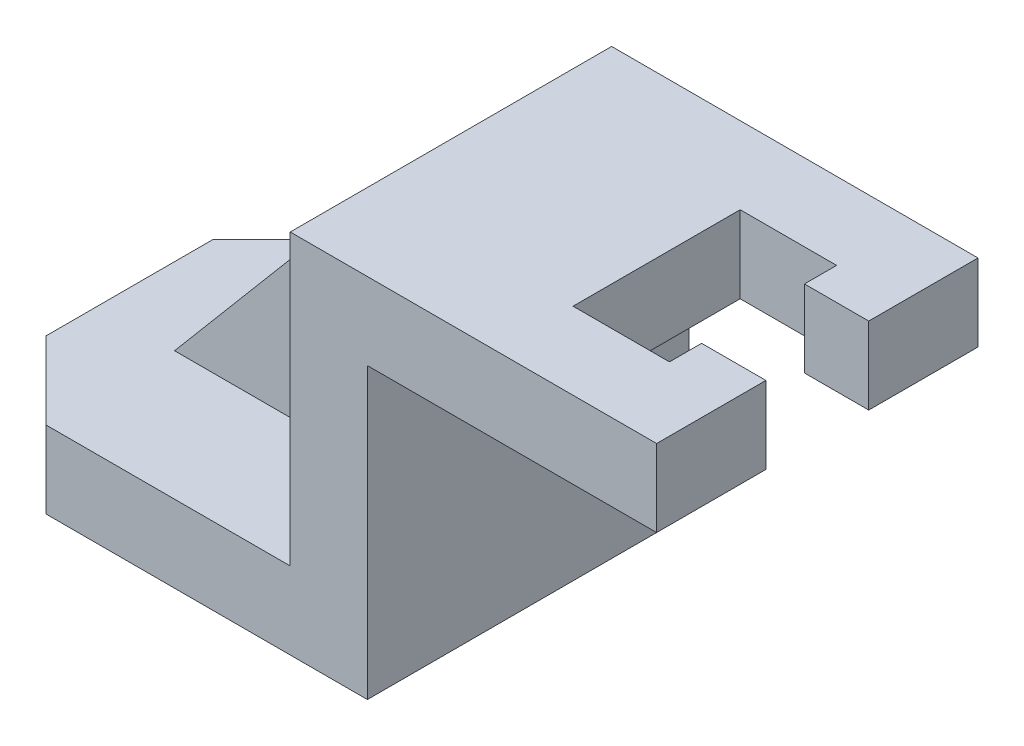
ISO-10303-21;
HEADER;
FILE_DESCRIPTION(('STEP AP214'),'2;1');
FILE_NAME('part.step','',(''),(''),'','','');
FILE_SCHEMA(('AUTOMOTIVE_DESIGN { 1 0 10303 214 1 1 1 1 }'));
ENDSEC;
DATA;
#1=APPLICATION_CONTEXT('core data for automotive mechanical design processes');
#2=APPLICATION_PROTOCOL_DEFINITION('international standard','automotive_design',2000,#1);
#3=PRODUCT_CONTEXT('',#1,'mechanical');
#4=PRODUCT('Part','Part','',(#3));
#5=PRODUCT_RELATED_PRODUCT_CATEGORY('part','',(#4));
#6=PRODUCT_DEFINITION_FORMATION('','',#4);
#7=PRODUCT_DEFINITION_CONTEXT('part definition',#1,'design');
#8=PRODUCT_DEFINITION('design','',#6,#7);
#9=PRODUCT_DEFINITION_SHAPE('','',#8);
#10=(LENGTH_UNIT() NAMED_UNIT(*) SI_UNIT(.MILLI.,.METRE.));
#11=(NAMED_UNIT(*) PLANE_ANGLE_UNIT() SI_UNIT($,.RADIAN.));
#12=(NAMED_UNIT(*) SI_UNIT($,.STERADIAN.) SOLID_ANGLE_UNIT());
#13=UNCERTAINTY_MEASURE_WITH_UNIT(LENGTH_MEASURE(1.E-05),#10,'distance_accuracy_value','');
#14=(GEOMETRIC_REPRESENTATION_CONTEXT(3) GLOBAL_UNCERTAINTY_ASSIGNED_CONTEXT((#13)) GLOBAL_UNIT_ASSIGNED_CONTEXT((#10,
#11,#12)) REPRESENTATION_CONTEXT('',''));
#15=CARTESIAN_POINT('',(0.,0.,0.));
#16=DIRECTION('',(0.,0.,1.));
#17=DIRECTION('',(1.,0.,0.));
#18=AXIS2_PLACEMENT_3D('',#15,#16,#17);
#19=CARTESIAN_POINT('',(50.,57.,20.));
#20=DIRECTION('',(-0.764029915846901,0.645180817826272,0.));
#21=DIRECTION('',(-0.645180817826272,-0.764029915846901,0.));
#22=AXIS2_PLACEMENT_3D('',#19,#20,#21);
#23=PLANE('',#22);
#24=DIRECTION('',(0.,0.,1.));
#25=VECTOR('',#24,1.);
#26=CARTESIAN_POINT('',(12.,12.,20.));
#27=LINE('',#26,#25);
#28=CARTESIAN_POINT('',(12.,12.,20.));
#29=VERTEX_POINT('',#28);
#30=CARTESIAN_POINT('',(12.,12.,30.));
#31=VERTEX_POINT('',#30);
#32=EDGE_CURVE('E225',#29,#31,#27,.T.);
#33=ORIENTED_EDGE('',*,*,#32,.T.);
#34=DIRECTION('',(-0.645180817826272,-0.764029915846901,0.));
#35=VECTOR('',#34,1.);
#36=CARTESIAN_POINT('',(12.,12.,30.));
#37=LINE('',#36,#35);
#38=CARTESIAN_POINT('',(50.,57.,30.));
#39=VERTEX_POINT('',#38);
#40=EDGE_CURVE('E200',#39,#31,#37,.T.);
#41=ORIENTED_EDGE('',*,*,#40,.F.);
#42=DIRECTION('',(0.,0.,-1.));
#43=VECTOR('',#42,1.);
#44=CARTESIAN_POINT('',(50.,57.,50.));
#45=LINE('',#44,#43);
#46=CARTESIAN_POINT('',(50.,57.,20.));
#47=VERTEX_POINT('',#46);
#48=EDGE_CURVE('E336',#39,#47,#45,.T.);
#49=ORIENTED_EDGE('',*,*,#48,.T.);
#50=DIRECTION('',(-0.645180817826272,-0.764029915846901,0.));
#51=VECTOR('',#50,1.);
#52=CARTESIAN_POINT('',(50.,57.,20.));
#53=LINE('',#52,#51);
#54=EDGE_CURVE('E196',#47,#29,#53,.T.);
#55=ORIENTED_EDGE('',*,*,#54,.T.);
#56=EDGE_LOOP('',(#33,#41,#49,#55));
#57=FACE_BOUND('',#56,.T.);
#58=ADVANCED_FACE('F44',(#57),#23,.T.);
#59=CARTESIAN_POINT('',(50.,57.,50.));
#60=DIRECTION('',(1.,0.,0.));
#61=DIRECTION('',(0.,0.,-1.));
#62=AXIS2_PLACEMENT_3D('',#59,#60,#61);
#63=PLANE('',#62);
#64=DIRECTION('',(0.,1.,0.));
#65=VECTOR('',#64,1.);
#66=CARTESIAN_POINT('',(50.,12.,20.));
#67=LINE('',#66,#65);
#68=CARTESIAN_POINT('',(50.,12.,20.));
#69=VERTEX_POINT('',#68);
#70=EDGE_CURVE('E218',#69,#47,#67,.T.);
#71=ORIENTED_EDGE('',*,*,#70,.T.);
#72=CARTESIAN_POINT('',(50.,57.,0.));
#73=VERTEX_POINT('',#72);
#74=EDGE_CURVE('E337',#47,#73,#45,.T.);
#75=ORIENTED_EDGE('',*,*,#74,.T.);
#76=DIRECTION('',(0.,-1.,0.));
#77=VECTOR('',#76,1.);
#78=CARTESIAN_POINT('',(50.,57.,0.));
#79=LINE('',#78,#77);
#80=CARTESIAN_POINT('',(50.,12.,0.));
#81=VERTEX_POINT('',#80);
#82=EDGE_CURVE('E330',#73,#81,#79,.T.);
#83=ORIENTED_EDGE('',*,*,#82,.T.);
#84=DIRECTION('',(0.,0.,-1.));
#85=VECTOR('',#84,1.);
#86=CARTESIAN_POINT('',(50.,12.,50.));
#87=LINE('',#86,#85);
#88=EDGE_CURVE('E331',#69,#81,#87,.T.);
#89=ORIENTED_EDGE('',*,*,#88,.F.);
#90=EDGE_LOOP('',(#71,#75,#83,#89));
#91=FACE_BOUND('',#90,.T.);
#92=ADVANCED_FACE('F390',(#91),#63,.F.);
#93=CARTESIAN_POINT('',(107.,45.,50.));
#94=DIRECTION('',(-1.,0.,0.));
#95=DIRECTION('',(0.,0.,1.));
#96=AXIS2_PLACEMENT_3D('',#93,#94,#95);
#97=PLANE('',#96);
#98=DIRECTION('',(0.,0.,-1.));
#99=VECTOR('',#98,1.);
#100=CARTESIAN_POINT('',(107.,45.,50.));
#101=LINE('',#100,#99);
#102=CARTESIAN_POINT('',(107.,45.,50.));
#103=VERTEX_POINT('',#102);
#104=CARTESIAN_POINT('',(107.,45.,33.));
#105=VERTEX_POINT('',#104);
#106=EDGE_CURVE('E344',#103,#105,#101,.T.);
#107=ORIENTED_EDGE('',*,*,#106,.T.);
#108=DIRECTION('',(0.,1.,0.));
#109=VECTOR('',#108,1.);
#110=CARTESIAN_POINT('',(107.,45.,33.));
#111=LINE('',#110,#109);
#112=CARTESIAN_POINT('',(107.,57.,33.));
#113=VERTEX_POINT('',#112);
#114=EDGE_CURVE('E262',#105,#113,#111,.T.);
#115=ORIENTED_EDGE('',*,*,#114,.T.);
#116=DIRECTION('',(0.,0.,-1.));
#117=VECTOR('',#116,1.);
#118=CARTESIAN_POINT('',(107.,57.,50.));
#119=LINE('',#118,#117);
#120=CARTESIAN_POINT('',(107.,57.,50.));
#121=VERTEX_POINT('',#120);
#122=EDGE_CURVE('E338',#121,#113,#119,.T.);
#123=ORIENTED_EDGE('',*,*,#122,.F.);
#124=DIRECTION('',(0.,1.,0.));
#125=VECTOR('',#124,1.);
#126=CARTESIAN_POINT('',(107.,45.,50.));
#127=LINE('',#126,#125);
#128=EDGE_CURVE('E310',#103,#121,#127,.T.);
#129=ORIENTED_EDGE('',*,*,#128,.F.);
#130=EDGE_LOOP('',(#107,#115,#123,#129));
#131=FACE_BOUND('',#130,.T.);
#132=ADVANCED_FACE('F398',(#131),#97,.F.);
#133=CARTESIAN_POINT('',(0.,0.,50.));
#134=DIRECTION('',(1.,0.,0.));
#135=DIRECTION('',(0.,0.,-1.));
#136=AXIS2_PLACEMENT_3D('',#133,#134,#135);
#137=PLANE('',#136);
#138=DIRECTION('',(0.,0.,-1.));
#139=VECTOR('',#138,1.);
#140=CARTESIAN_POINT('',(0.,0.,50.));
#141=LINE('',#140,#139);
#142=CARTESIAN_POINT('',(0.,0.,38.));
#143=VERTEX_POINT('',#142);
#144=CARTESIAN_POINT('',(0.,0.,12.));
#145=VERTEX_POINT('',#144);
#146=EDGE_CURVE('E11',#143,#145,#141,.T.);
#147=ORIENTED_EDGE('',*,*,#146,.F.);
#148=DIRECTION('',(0.,1.,0.));
#149=VECTOR('',#148,1.);
#150=CARTESIAN_POINT('',(0.,0.,38.));
#151=LINE('',#150,#149);
#152=CARTESIAN_POINT('',(0.,12.,38.));
#153=VERTEX_POINT('',#152);
#154=EDGE_CURVE('E288',#143,#153,#151,.T.);
#155=ORIENTED_EDGE('',*,*,#154,.T.);
#156=DIRECTION('',(0.,0.,-1.));
#157=VECTOR('',#156,1.);
#158=CARTESIAN_POINT('',(0.,12.,50.));
#159=LINE('',#158,#157);
#160=CARTESIAN_POINT('',(0.,12.,12.));
#161=VERTEX_POINT('',#160);
#162=EDGE_CURVE('E314',#153,#161,#159,.T.);
#163=ORIENTED_EDGE('',*,*,#162,.T.);
#164=DIRECTION('',(0.,1.,0.));
#165=VECTOR('',#164,1.);
#166=CARTESIAN_POINT('',(0.,0.,12.));
#167=LINE('',#166,#165);
#168=EDGE_CURVE('E299',#145,#161,#167,.T.);
#169=ORIENTED_EDGE('',*,*,#168,.F.);
#170=EDGE_LOOP('',(#147,#155,#163,#169));
#171=FACE_BOUND('',#170,.T.);
#172=ADVANCED_FACE('F50',(#171),#137,.F.);
#173=CARTESIAN_POINT('',(12.,0.,50.));
#174=DIRECTION('',(0.,1.,0.));
#175=DIRECTION('',(0.,0.,1.));
#176=AXIS2_PLACEMENT_3D('',#173,#174,#175);
#177=PLANE('',#176);
#178=DIRECTION('',(1.,0.,0.));
#179=VECTOR('',#178,1.);
#180=CARTESIAN_POINT('',(0.,0.,50.));
#181=LINE('',#180,#179);
#182=CARTESIAN_POINT('',(12.,0.,50.));
#183=VERTEX_POINT('',#182);
#184=CARTESIAN_POINT('',(62.,0.,50.));
#185=VERTEX_POINT('',#184);
#186=EDGE_CURVE('E305',#183,#185,#181,.T.);
#187=ORIENTED_EDGE('',*,*,#186,.F.);
#188=DIRECTION('',(-0.707106781186548,0.,-0.707106781186548));
#189=VECTOR('',#188,1.);
#190=CARTESIAN_POINT('',(12.,0.,50.));
#191=LINE('',#190,#189);
#192=EDGE_CURVE('E282',#183,#143,#191,.T.);
#193=ORIENTED_EDGE('',*,*,#192,.T.);
#194=ORIENTED_EDGE('',*,*,#146,.T.);
#195=DIRECTION('',(0.707106781186548,0.,-0.707106781186548));
#196=VECTOR('',#195,1.);
#197=CARTESIAN_POINT('',(0.,0.,12.));
#198=LINE('',#197,#196);
#199=CARTESIAN_POINT('',(12.,0.,0.));
#200=VERTEX_POINT('',#199);
#201=EDGE_CURVE('E294',#145,#200,#198,.T.);
#202=ORIENTED_EDGE('',*,*,#201,.T.);
#203=DIRECTION('',(1.,0.,0.));
#204=VECTOR('',#203,1.);
#205=CARTESIAN_POINT('',(12.,0.,0.));
#206=LINE('',#205,#204);
#207=CARTESIAN_POINT('',(62.,0.,0.));
#208=VERTEX_POINT('',#207);
#209=EDGE_CURVE('E292',#200,#208,#206,.T.);
#210=ORIENTED_EDGE('',*,*,#209,.T.);
#211=DIRECTION('',(0.,0.,-1.));
#212=VECTOR('',#211,1.);
#213=CARTESIAN_POINT('',(62.,0.,50.));
#214=LINE('',#213,#212);
#215=EDGE_CURVE('E52',#185,#208,#214,.T.);
#216=ORIENTED_EDGE('',*,*,#215,.F.);
#217=EDGE_LOOP('',(#187,#193,#194,#202,#210,#216));
#218=FACE_BOUND('',#217,.T.);
#219=ADVANCED_FACE('F372',(#218),#177,.F.);
#220=CARTESIAN_POINT('',(62.,0.,50.));
#221=DIRECTION('',(-1.,0.,0.));
#222=DIRECTION('',(0.,0.,1.));
#223=AXIS2_PLACEMENT_3D('',#220,#221,#222);
#224=PLANE('',#223);
#225=DIRECTION('',(0.,1.,0.));
#226=VECTOR('',#225,1.);
#227=CARTESIAN_POINT('',(62.,0.,0.));
#228=LINE('',#227,#226);
#229=CARTESIAN_POINT('',(62.,45.,0.));
#230=VERTEX_POINT('',#229);
#231=EDGE_CURVE('E316',#208,#230,#228,.T.);
#232=ORIENTED_EDGE('',*,*,#231,.T.);
#233=DIRECTION('',(0.,0.,-1.));
#234=VECTOR('',#233,1.);
#235=CARTESIAN_POINT('',(62.,45.,50.));
#236=LINE('',#235,#234);
#237=CARTESIAN_POINT('',(62.,45.,50.));
#238=VERTEX_POINT('',#237);
#239=EDGE_CURVE('E350',#238,#230,#236,.T.);
#240=ORIENTED_EDGE('',*,*,#239,.F.);
#241=DIRECTION('',(0.,1.,0.));
#242=VECTOR('',#241,1.);
#243=CARTESIAN_POINT('',(62.,0.,50.));
#244=LINE('',#243,#242);
#245=EDGE_CURVE('E304',#185,#238,#244,.T.);
#246=ORIENTED_EDGE('',*,*,#245,.F.);
#247=ORIENTED_EDGE('',*,*,#215,.T.);
#248=EDGE_LOOP('',(#232,#240,#246,#247));
#249=FACE_BOUND('',#248,.T.);
#250=ADVANCED_FACE('F351',(#249),#224,.F.);
#251=CARTESIAN_POINT('',(62.,45.,50.));
#252=DIRECTION('',(0.,1.,0.));
#253=DIRECTION('',(0.,0.,1.));
#254=AXIS2_PLACEMENT_3D('',#251,#252,#253);
#255=PLANE('',#254);
#256=DIRECTION('',(0.,0.,-1.));
#257=VECTOR('',#256,1.);
#258=CARTESIAN_POINT('',(97.,45.,33.));
#259=LINE('',#258,#257);
#260=CARTESIAN_POINT('',(97.,45.,38.));
#261=VERTEX_POINT('',#260);
#262=CARTESIAN_POINT('',(97.,45.,33.));
#263=VERTEX_POINT('',#262);
#264=EDGE_CURVE('E242',#261,#263,#259,.T.);
#265=ORIENTED_EDGE('',*,*,#264,.T.);
#266=DIRECTION('',(1.,0.,0.));
#267=VECTOR('',#266,1.);
#268=CARTESIAN_POINT('',(107.,45.,33.));
#269=LINE('',#268,#267);
#270=EDGE_CURVE('E241',#263,#105,#269,.T.);
#271=ORIENTED_EDGE('',*,*,#270,.T.);
#272=ORIENTED_EDGE('',*,*,#106,.F.);
#273=DIRECTION('',(1.,0.,0.));
#274=VECTOR('',#273,1.);
#275=CARTESIAN_POINT('',(62.,45.,50.));
#276=LINE('',#275,#274);
#277=EDGE_CURVE('E307',#238,#103,#276,.T.);
#278=ORIENTED_EDGE('',*,*,#277,.F.);
#279=ORIENTED_EDGE('',*,*,#239,.T.);
#280=DIRECTION('',(1.,0.,0.));
#281=VECTOR('',#280,1.);
#282=CARTESIAN_POINT('',(62.,45.,0.));
#283=LINE('',#282,#281);
#284=CARTESIAN_POINT('',(107.,45.,0.));
#285=VERTEX_POINT('',#284);
#286=EDGE_CURVE('E318',#230,#285,#283,.T.);
#287=ORIENTED_EDGE('',*,*,#286,.T.);
#288=CARTESIAN_POINT('',(107.,45.,17.));
#289=VERTEX_POINT('',#288);
#290=EDGE_CURVE('E343',#289,#285,#101,.T.);
#291=ORIENTED_EDGE('',*,*,#290,.F.);
#292=DIRECTION('',(-1.,0.,0.));
#293=VECTOR('',#292,1.);
#294=CARTESIAN_POINT('',(107.,45.,17.));
#295=LINE('',#294,#293);
#296=CARTESIAN_POINT('',(97.,45.,17.));
#297=VERTEX_POINT('',#296);
#298=EDGE_CURVE('E223',#289,#297,#295,.T.);
#299=ORIENTED_EDGE('',*,*,#298,.T.);
#300=DIRECTION('',(0.,0.,-1.));
#301=VECTOR('',#300,1.);
#302=CARTESIAN_POINT('',(97.,45.,12.));
#303=LINE('',#302,#301);
#304=CARTESIAN_POINT('',(97.,45.,12.));
#305=VERTEX_POINT('',#304);
#306=EDGE_CURVE('E230',#297,#305,#303,.T.);
#307=ORIENTED_EDGE('',*,*,#306,.T.);
#308=DIRECTION('',(-1.,0.,0.));
#309=VECTOR('',#308,1.);
#310=CARTESIAN_POINT('',(82.,45.,12.));
#311=LINE('',#310,#309);
#312=CARTESIAN_POINT('',(82.,45.,12.));
#313=VERTEX_POINT('',#312);
#314=EDGE_CURVE('E235',#305,#313,#311,.T.);
#315=ORIENTED_EDGE('',*,*,#314,.T.);
#316=DIRECTION('',(0.,0.,1.));
#317=VECTOR('',#316,1.);
#318=CARTESIAN_POINT('',(82.,45.,38.));
#319=LINE('',#318,#317);
#320=CARTESIAN_POINT('',(82.,45.,38.));
#321=VERTEX_POINT('',#320);
#322=EDGE_CURVE('E231',#313,#321,#319,.T.);
#323=ORIENTED_EDGE('',*,*,#322,.T.);
#324=DIRECTION('',(1.,0.,0.));
#325=VECTOR('',#324,1.);
#326=CARTESIAN_POINT('',(97.,45.,38.));
#327=LINE('',#326,#325);
#328=EDGE_CURVE('E236',#321,#261,#327,.T.);
#329=ORIENTED_EDGE('',*,*,#328,.T.);
#330=EDGE_LOOP('',(#265,#271,#272,#278,#279,#287,#291,#299,#307,#315,#323,#329));
#331=FACE_BOUND('',#330,.T.);
#332=ADVANCED_FACE('F368',(#331),#255,.F.);
#333=CARTESIAN_POINT('',(107.,57.,17.));
#334=VERTEX_POINT('',#333);
#335=CARTESIAN_POINT('',(107.,57.,0.));
#336=VERTEX_POINT('',#335);
#337=EDGE_CURVE('E340',#334,#336,#119,.T.);
#338=ORIENTED_EDGE('',*,*,#337,.F.);
#339=DIRECTION('',(0.,1.,0.));
#340=VECTOR('',#339,1.);
#341=CARTESIAN_POINT('',(107.,45.,17.));
#342=LINE('',#341,#340);
#343=EDGE_CURVE('E68',#289,#334,#342,.T.);
#344=ORIENTED_EDGE('',*,*,#343,.F.);
#345=ORIENTED_EDGE('',*,*,#290,.T.);
#346=DIRECTION('',(0.,1.,0.));
#347=VECTOR('',#346,1.);
#348=CARTESIAN_POINT('',(107.,45.,0.));
#349=LINE('',#348,#347);
#350=EDGE_CURVE('E321',#285,#336,#349,.T.);
#351=ORIENTED_EDGE('',*,*,#350,.T.);
#352=EDGE_LOOP('',(#338,#344,#345,#351));
#353=FACE_BOUND('',#352,.T.);
#354=ADVANCED_FACE('F393',(#353),#97,.F.);
#355=CARTESIAN_POINT('',(107.,57.,50.));
#356=DIRECTION('',(0.,-1.,0.));
#357=DIRECTION('',(0.,0.,-1.));
#358=AXIS2_PLACEMENT_3D('',#355,#356,#357);
#359=PLANE('',#358);
#360=ORIENTED_EDGE('',*,*,#122,.T.);
#361=DIRECTION('',(1.,0.,0.));
#362=VECTOR('',#361,1.);
#363=CARTESIAN_POINT('',(107.,57.,33.));
#364=LINE('',#363,#362);
#365=CARTESIAN_POINT('',(97.,57.,33.));
#366=VERTEX_POINT('',#365);
#367=EDGE_CURVE('E226',#366,#113,#364,.T.);
#368=ORIENTED_EDGE('',*,*,#367,.F.);
#369=DIRECTION('',(0.,0.,-1.));
#370=VECTOR('',#369,1.);
#371=CARTESIAN_POINT('',(97.,57.,33.));
#372=LINE('',#371,#370);
#373=CARTESIAN_POINT('',(97.,57.,38.));
#374=VERTEX_POINT('',#373);
#375=EDGE_CURVE('E257',#374,#366,#372,.T.);
#376=ORIENTED_EDGE('',*,*,#375,.F.);
#377=DIRECTION('',(1.,0.,0.));
#378=VECTOR('',#377,1.);
#379=CARTESIAN_POINT('',(97.,57.,38.));
#380=LINE('',#379,#378);
#381=CARTESIAN_POINT('',(82.,57.,38.));
#382=VERTEX_POINT('',#381);
#383=EDGE_CURVE('E260',#382,#374,#380,.T.);
#384=ORIENTED_EDGE('',*,*,#383,.F.);
#385=DIRECTION('',(0.,0.,1.));
#386=VECTOR('',#385,1.);
#387=CARTESIAN_POINT('',(82.,57.,38.));
#388=LINE('',#387,#386);
#389=CARTESIAN_POINT('',(82.,57.,12.));
#390=VERTEX_POINT('',#389);
#391=EDGE_CURVE('E255',#390,#382,#388,.T.);
#392=ORIENTED_EDGE('',*,*,#391,.F.);
#393=DIRECTION('',(-1.,0.,0.));
#394=VECTOR('',#393,1.);
#395=CARTESIAN_POINT('',(82.,57.,12.));
#396=LINE('',#395,#394);
#397=CARTESIAN_POINT('',(97.,57.,12.));
#398=VERTEX_POINT('',#397);
#399=EDGE_CURVE('E253',#398,#390,#396,.T.);
#400=ORIENTED_EDGE('',*,*,#399,.F.);
#401=DIRECTION('',(0.,0.,-1.));
#402=VECTOR('',#401,1.);
#403=CARTESIAN_POINT('',(97.,57.,12.));
#404=LINE('',#403,#402);
#405=CARTESIAN_POINT('',(97.,57.,17.));
#406=VERTEX_POINT('',#405);
#407=EDGE_CURVE('E248',#406,#398,#404,.T.);
#408=ORIENTED_EDGE('',*,*,#407,.F.);
#409=DIRECTION('',(-1.,0.,0.));
#410=VECTOR('',#409,1.);
#411=CARTESIAN_POINT('',(107.,57.,17.));
#412=LINE('',#411,#410);
#413=EDGE_CURVE('E221',#334,#406,#412,.T.);
#414=ORIENTED_EDGE('',*,*,#413,.F.);
#415=ORIENTED_EDGE('',*,*,#337,.T.);
#416=DIRECTION('',(-1.,0.,0.));
#417=VECTOR('',#416,1.);
#418=CARTESIAN_POINT('',(107.,57.,0.));
#419=LINE('',#418,#417);
#420=EDGE_CURVE('E322',#336,#73,#419,.T.);
#421=ORIENTED_EDGE('',*,*,#420,.T.);
#422=ORIENTED_EDGE('',*,*,#74,.F.);
#423=ORIENTED_EDGE('',*,*,#48,.F.);
#424=CARTESIAN_POINT('',(50.,57.,50.));
#425=VERTEX_POINT('',#424);
#426=EDGE_CURVE('E201',#425,#39,#45,.T.);
#427=ORIENTED_EDGE('',*,*,#426,.F.);
#428=DIRECTION('',(-1.,0.,0.));
#429=VECTOR('',#428,1.);
#430=CARTESIAN_POINT('',(107.,57.,50.));
#431=LINE('',#430,#429);
#432=EDGE_CURVE('E313',#121,#425,#431,.T.);
#433=ORIENTED_EDGE('',*,*,#432,.F.);
#434=EDGE_LOOP('',(#360,#368,#376,#384,#392,#400,#408,#414,#415,#421,#422,#423,#427,#433));
#435=FACE_BOUND('',#434,.T.);
#436=ADVANCED_FACE('F392',(#435),#359,.F.);
#437=CARTESIAN_POINT('',(0.,12.,50.));
#438=DIRECTION('',(0.,-1.,0.));
#439=DIRECTION('',(0.,0.,-1.));
#440=AXIS2_PLACEMENT_3D('',#437,#438,#439);
#441=PLANE('',#440);
#442=DIRECTION('',(-0.707106781186548,0.,-0.707106781186548));
#443=VECTOR('',#442,1.);
#444=CARTESIAN_POINT('',(12.,12.,50.));
#445=LINE('',#444,#443);
#446=CARTESIAN_POINT('',(12.,12.,50.));
#447=VERTEX_POINT('',#446);
#448=EDGE_CURVE('E283',#447,#153,#445,.T.);
#449=ORIENTED_EDGE('',*,*,#448,.F.);
#450=DIRECTION('',(1.,0.,0.));
#451=VECTOR('',#450,1.);
#452=CARTESIAN_POINT('',(50.,12.,50.));
#453=LINE('',#452,#451);
#454=CARTESIAN_POINT('',(50.,12.,50.));
#455=VERTEX_POINT('',#454);
#456=EDGE_CURVE('E191',#447,#455,#453,.T.);
#457=ORIENTED_EDGE('',*,*,#456,.T.);
#458=DIRECTION('',(0.,0.,1.));
#459=VECTOR('',#458,1.);
#460=CARTESIAN_POINT('',(50.,12.,30.));
#461=LINE('',#460,#459);
#462=CARTESIAN_POINT('',(50.,12.,30.));
#463=VERTEX_POINT('',#462);
#464=EDGE_CURVE('E188',#463,#455,#461,.T.);
#465=ORIENTED_EDGE('',*,*,#464,.F.);
#466=DIRECTION('',(1.,0.,0.));
#467=VECTOR('',#466,1.);
#468=CARTESIAN_POINT('',(50.,12.,30.));
#469=LINE('',#468,#467);
#470=EDGE_CURVE('E194',#31,#463,#469,.T.);
#471=ORIENTED_EDGE('',*,*,#470,.F.);
#472=ORIENTED_EDGE('',*,*,#32,.F.);
#473=DIRECTION('',(1.,0.,0.));
#474=VECTOR('',#473,1.);
#475=CARTESIAN_POINT('',(12.,12.,20.));
#476=LINE('',#475,#474);
#477=EDGE_CURVE('E216',#29,#69,#476,.T.);
#478=ORIENTED_EDGE('',*,*,#477,.T.);
#479=ORIENTED_EDGE('',*,*,#88,.T.);
#480=DIRECTION('',(-1.,0.,0.));
#481=VECTOR('',#480,1.);
#482=CARTESIAN_POINT('',(0.,12.,0.));
#483=LINE('',#482,#481);
#484=CARTESIAN_POINT('',(12.,12.,0.));
#485=VERTEX_POINT('',#484);
#486=EDGE_CURVE('E301',#81,#485,#483,.T.);
#487=ORIENTED_EDGE('',*,*,#486,.T.);
#488=DIRECTION('',(0.707106781186548,0.,-0.707106781186548));
#489=VECTOR('',#488,1.);
#490=CARTESIAN_POINT('',(0.,12.,12.));
#491=LINE('',#490,#489);
#492=EDGE_CURVE('E270',#161,#485,#491,.T.);
#493=ORIENTED_EDGE('',*,*,#492,.F.);
#494=ORIENTED_EDGE('',*,*,#162,.F.);
#495=EDGE_LOOP('',(#449,#457,#465,#471,#472,#478,#479,#487,#493,#494));
#496=FACE_BOUND('',#495,.T.);
#497=ADVANCED_FACE('F195',(#496),#441,.F.);
#498=CARTESIAN_POINT('',(0.,0.,50.));
#499=DIRECTION('',(0.,0.,-1.));
#500=DIRECTION('',(-1.,0.,0.));
#501=AXIS2_PLACEMENT_3D('',#498,#499,#500);
#502=PLANE('',#501);
#503=DIRECTION('',(0.,1.,0.));
#504=VECTOR('',#503,1.);
#505=CARTESIAN_POINT('',(50.,57.,50.));
#506=LINE('',#505,#504);
#507=EDGE_CURVE('E208',#455,#425,#506,.T.);
#508=ORIENTED_EDGE('',*,*,#507,.F.);
#509=ORIENTED_EDGE('',*,*,#456,.F.);
#510=DIRECTION('',(0.,1.,0.));
#511=VECTOR('',#510,1.);
#512=CARTESIAN_POINT('',(12.,0.,50.));
#513=LINE('',#512,#511);
#514=EDGE_CURVE('E281',#183,#447,#513,.T.);
#515=ORIENTED_EDGE('',*,*,#514,.F.);
#516=ORIENTED_EDGE('',*,*,#186,.T.);
#517=ORIENTED_EDGE('',*,*,#245,.T.);
#518=ORIENTED_EDGE('',*,*,#277,.T.);
#519=ORIENTED_EDGE('',*,*,#128,.T.);
#520=ORIENTED_EDGE('',*,*,#432,.T.);
#521=EDGE_LOOP('',(#508,#509,#515,#516,#517,#518,#519,#520));
#522=FACE_BOUND('',#521,.T.);
#523=ADVANCED_FACE('F371',(#522),#502,.F.);
#524=CARTESIAN_POINT('',(0.,0.,0.));
#525=DIRECTION('',(0.,0.,-1.));
#526=DIRECTION('',(-1.,0.,0.));
#527=AXIS2_PLACEMENT_3D('',#524,#525,#526);
#528=PLANE('',#527);
#529=DIRECTION('',(0.,1.,0.));
#530=VECTOR('',#529,1.);
#531=CARTESIAN_POINT('',(12.,0.,0.));
#532=LINE('',#531,#530);
#533=EDGE_CURVE('E290',#200,#485,#532,.T.);
#534=ORIENTED_EDGE('',*,*,#533,.T.);
#535=ORIENTED_EDGE('',*,*,#486,.F.);
#536=ORIENTED_EDGE('',*,*,#82,.F.);
#537=ORIENTED_EDGE('',*,*,#420,.F.);
#538=ORIENTED_EDGE('',*,*,#350,.F.);
#539=ORIENTED_EDGE('',*,*,#286,.F.);
#540=ORIENTED_EDGE('',*,*,#231,.F.);
#541=ORIENTED_EDGE('',*,*,#209,.F.);
#542=EDGE_LOOP('',(#534,#535,#536,#537,#538,#539,#540,#541));
#543=FACE_BOUND('',#542,.T.);
#544=ADVANCED_FACE('F363',(#543),#528,.T.);
#545=CARTESIAN_POINT('',(0.,0.,12.));
#546=DIRECTION('',(0.707106781186547,0.,0.707106781186547));
#547=DIRECTION('',(0.707106781186548,0.,-0.707106781186548));
#548=AXIS2_PLACEMENT_3D('',#545,#546,#547);
#549=PLANE('',#548);
#550=ORIENTED_EDGE('',*,*,#492,.T.);
#551=ORIENTED_EDGE('',*,*,#533,.F.);
#552=ORIENTED_EDGE('',*,*,#201,.F.);
#553=ORIENTED_EDGE('',*,*,#168,.T.);
#554=EDGE_LOOP('',(#550,#551,#552,#553));
#555=FACE_BOUND('',#554,.T.);
#556=ADVANCED_FACE('F385',(#555),#549,.F.);
#557=CARTESIAN_POINT('',(12.,0.,50.));
#558=DIRECTION('',(0.707106781186547,0.,-0.707106781186547));
#559=DIRECTION('',(-0.707106781186548,0.,-0.707106781186548));
#560=AXIS2_PLACEMENT_3D('',#557,#558,#559);
#561=PLANE('',#560);
#562=ORIENTED_EDGE('',*,*,#448,.T.);
#563=ORIENTED_EDGE('',*,*,#154,.F.);
#564=ORIENTED_EDGE('',*,*,#192,.F.);
#565=ORIENTED_EDGE('',*,*,#514,.T.);
#566=EDGE_LOOP('',(#562,#563,#564,#565));
#567=FACE_BOUND('',#566,.T.);
#568=ADVANCED_FACE('F424',(#567),#561,.F.);
#569=CARTESIAN_POINT('',(107.,45.,33.));
#570=DIRECTION('',(0.,0.,1.));
#571=DIRECTION('',(1.,0.,0.));
#572=AXIS2_PLACEMENT_3D('',#569,#570,#571);
#573=PLANE('',#572);
#574=ORIENTED_EDGE('',*,*,#367,.T.);
#575=ORIENTED_EDGE('',*,*,#114,.F.);
#576=ORIENTED_EDGE('',*,*,#270,.F.);
#577=DIRECTION('',(0.,1.,0.));
#578=VECTOR('',#577,1.);
#579=CARTESIAN_POINT('',(97.,45.,33.));
#580=LINE('',#579,#578);
#581=EDGE_CURVE('E268',#263,#366,#580,.T.);
#582=ORIENTED_EDGE('',*,*,#581,.T.);
#583=EDGE_LOOP('',(#574,#575,#576,#582));
#584=FACE_BOUND('',#583,.T.);
#585=ADVANCED_FACE('F419',(#584),#573,.F.);
#586=CARTESIAN_POINT('',(97.,45.,33.));
#587=DIRECTION('',(1.,0.,0.));
#588=DIRECTION('',(0.,0.,-1.));
#589=AXIS2_PLACEMENT_3D('',#586,#587,#588);
#590=PLANE('',#589);
#591=ORIENTED_EDGE('',*,*,#375,.T.);
#592=ORIENTED_EDGE('',*,*,#581,.F.);
#593=ORIENTED_EDGE('',*,*,#264,.F.);
#594=DIRECTION('',(0.,1.,0.));
#595=VECTOR('',#594,1.);
#596=CARTESIAN_POINT('',(97.,45.,38.));
#597=LINE('',#596,#595);
#598=EDGE_CURVE('E269',#261,#374,#597,.T.);
#599=ORIENTED_EDGE('',*,*,#598,.T.);
#600=EDGE_LOOP('',(#591,#592,#593,#599));
#601=FACE_BOUND('',#600,.T.);
#602=ADVANCED_FACE('F421',(#601),#590,.F.);
#603=CARTESIAN_POINT('',(97.,45.,38.));
#604=DIRECTION('',(0.,0.,1.));
#605=DIRECTION('',(1.,0.,0.));
#606=AXIS2_PLACEMENT_3D('',#603,#604,#605);
#607=PLANE('',#606);
#608=ORIENTED_EDGE('',*,*,#383,.T.);
#609=ORIENTED_EDGE('',*,*,#598,.F.);
#610=ORIENTED_EDGE('',*,*,#328,.F.);
#611=DIRECTION('',(0.,1.,0.));
#612=VECTOR('',#611,1.);
#613=CARTESIAN_POINT('',(82.,45.,38.));
#614=LINE('',#613,#612);
#615=EDGE_CURVE('E275',#321,#382,#614,.T.);
#616=ORIENTED_EDGE('',*,*,#615,.T.);
#617=EDGE_LOOP('',(#608,#609,#610,#616));
#618=FACE_BOUND('',#617,.T.);
#619=ADVANCED_FACE('F428',(#618),#607,.F.);
#620=CARTESIAN_POINT('',(82.,45.,38.));
#621=DIRECTION('',(-1.,0.,0.));
#622=DIRECTION('',(0.,0.,1.));
#623=AXIS2_PLACEMENT_3D('',#620,#621,#622);
#624=PLANE('',#623);
#625=ORIENTED_EDGE('',*,*,#391,.T.);
#626=ORIENTED_EDGE('',*,*,#615,.F.);
#627=ORIENTED_EDGE('',*,*,#322,.F.);
#628=DIRECTION('',(0.,1.,0.));
#629=VECTOR('',#628,1.);
#630=CARTESIAN_POINT('',(82.,45.,12.));
#631=LINE('',#630,#629);
#632=EDGE_CURVE('E273',#313,#390,#631,.T.);
#633=ORIENTED_EDGE('',*,*,#632,.T.);
#634=EDGE_LOOP('',(#625,#626,#627,#633));
#635=FACE_BOUND('',#634,.T.);
#636=ADVANCED_FACE('F435',(#635),#624,.F.);
#637=CARTESIAN_POINT('',(82.,45.,12.));
#638=DIRECTION('',(0.,0.,-1.));
#639=DIRECTION('',(-1.,0.,0.));
#640=AXIS2_PLACEMENT_3D('',#637,#638,#639);
#641=PLANE('',#640);
#642=ORIENTED_EDGE('',*,*,#399,.T.);
#643=ORIENTED_EDGE('',*,*,#632,.F.);
#644=ORIENTED_EDGE('',*,*,#314,.F.);
#645=DIRECTION('',(0.,1.,0.));
#646=VECTOR('',#645,1.);
#647=CARTESIAN_POINT('',(97.,45.,12.));
#648=LINE('',#647,#646);
#649=EDGE_CURVE('E277',#305,#398,#648,.T.);
#650=ORIENTED_EDGE('',*,*,#649,.T.);
#651=EDGE_LOOP('',(#642,#643,#644,#650));
#652=FACE_BOUND('',#651,.T.);
#653=ADVANCED_FACE('F436',(#652),#641,.F.);
#654=CARTESIAN_POINT('',(97.,45.,12.));
#655=DIRECTION('',(1.,0.,0.));
#656=DIRECTION('',(0.,0.,-1.));
#657=AXIS2_PLACEMENT_3D('',#654,#655,#656);
#658=PLANE('',#657);
#659=ORIENTED_EDGE('',*,*,#407,.T.);
#660=ORIENTED_EDGE('',*,*,#649,.F.);
#661=ORIENTED_EDGE('',*,*,#306,.F.);
#662=DIRECTION('',(0.,1.,0.));
#663=VECTOR('',#662,1.);
#664=CARTESIAN_POINT('',(97.,45.,17.));
#665=LINE('',#664,#663);
#666=EDGE_CURVE('E279',#297,#406,#665,.T.);
#667=ORIENTED_EDGE('',*,*,#666,.T.);
#668=EDGE_LOOP('',(#659,#660,#661,#667));
#669=FACE_BOUND('',#668,.T.);
#670=ADVANCED_FACE('F439',(#669),#658,.F.);
#671=CARTESIAN_POINT('',(107.,45.,17.));
#672=DIRECTION('',(0.,0.,-1.));
#673=DIRECTION('',(-1.,0.,0.));
#674=AXIS2_PLACEMENT_3D('',#671,#672,#673);
#675=PLANE('',#674);
#676=ORIENTED_EDGE('',*,*,#413,.T.);
#677=ORIENTED_EDGE('',*,*,#666,.F.);
#678=ORIENTED_EDGE('',*,*,#298,.F.);
#679=ORIENTED_EDGE('',*,*,#343,.T.);
#680=EDGE_LOOP('',(#676,#677,#678,#679));
#681=FACE_BOUND('',#680,.T.);
#682=ADVANCED_FACE('F441',(#681),#675,.F.);
#683=CARTESIAN_POINT('',(0.,0.,20.));
#684=DIRECTION('',(0.,0.,1.));
#685=DIRECTION('',(1.,0.,0.));
#686=AXIS2_PLACEMENT_3D('',#683,#684,#685);
#687=PLANE('',#686);
#688=ORIENTED_EDGE('',*,*,#54,.F.);
#689=ORIENTED_EDGE('',*,*,#70,.F.);
#690=ORIENTED_EDGE('',*,*,#477,.F.);
#691=EDGE_LOOP('',(#688,#689,#690));
#692=FACE_BOUND('',#691,.T.);
#693=ADVANCED_FACE('F416',(#692),#687,.F.);
#694=CARTESIAN_POINT('',(50.,57.,30.));
#695=DIRECTION('',(1.,0.,0.));
#696=DIRECTION('',(0.,0.,-1.));
#697=AXIS2_PLACEMENT_3D('',#694,#695,#696);
#698=PLANE('',#697);
#699=ORIENTED_EDGE('',*,*,#507,.T.);
#700=ORIENTED_EDGE('',*,*,#426,.T.);
#701=DIRECTION('',(0.,1.,0.));
#702=VECTOR('',#701,1.);
#703=CARTESIAN_POINT('',(50.,57.,30.));
#704=LINE('',#703,#702);
#705=EDGE_CURVE('E58',#463,#39,#704,.T.);
#706=ORIENTED_EDGE('',*,*,#705,.F.);
#707=ORIENTED_EDGE('',*,*,#464,.T.);
#708=EDGE_LOOP('',(#699,#700,#706,#707));
#709=FACE_BOUND('',#708,.T.);
#710=ADVANCED_FACE('F203',(#709),#698,.F.);
#711=CARTESIAN_POINT('',(0.,0.,30.));
#712=DIRECTION('',(0.,0.,1.));
#713=DIRECTION('',(1.,0.,0.));
#714=AXIS2_PLACEMENT_3D('',#711,#712,#713);
#715=PLANE('',#714);
#716=ORIENTED_EDGE('',*,*,#470,.T.);
#717=ORIENTED_EDGE('',*,*,#705,.T.);
#718=ORIENTED_EDGE('',*,*,#40,.T.);
#719=EDGE_LOOP('',(#716,#717,#718));
#720=FACE_BOUND('',#719,.T.);
#721=ADVANCED_FACE('F206',(#720),#715,.T.);
#722=CLOSED_SHELL('',(#58,#92,#132,#172,#219,#250,#332,#354,#436,#497,#523,#544,#556,#568,#585,
#602,#619,#636,#653,#670,#682,#693,#710,#721));
#723=MANIFOLD_SOLID_BREP('B2',#722);
#724=ADVANCED_BREP_SHAPE_REPRESENTATION('',(#18,#723),#14);
#725=SHAPE_DEFINITION_REPRESENTATION(#9,#724);
ENDSEC;
END-ISO-10303-21;
